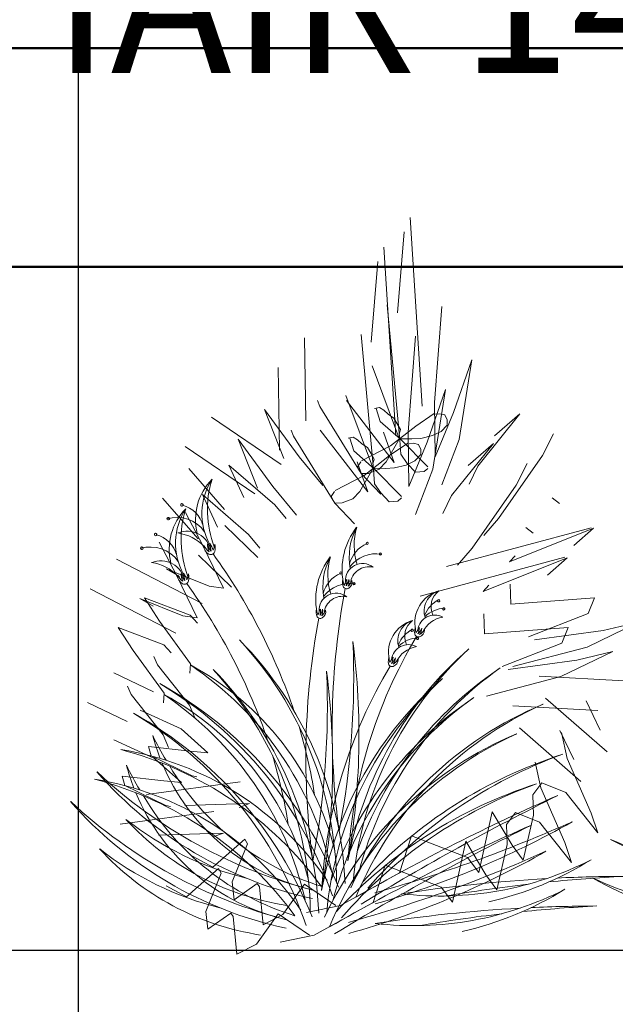
# Model space of a CAD drawing. Units: inches. Extents: x 89 to 490, y -59 to 378.
# Tile 3 of 20: x 275 to 300, y -26 to 15. Entities that reach past the tile are written whole.
import ezdxf

# ---------------------------------------------------------------- set-up
doc = ezdxf.new("R2010")
doc.units = ezdxf.units.IN
doc.header["$MEASUREMENT"] = 0
for name, color, linetype, lineweight in [('A-ANNO-DIMS', 2, 'Continuous', 18), ('L-PLNT', 94, 'Continuous', 18), ('L-PLNT-EDGE', 31, 'Continuous', 25), ('Outer Walls', 12, 'Continuous', 50)]:
    doc.layers.add(name, color=color, linetype=linetype, lineweight=lineweight)
doc.layers.add('fl', color=73, linetype='Continuous', lineweight=9, true_color=0xa3d166)
doc.styles.get("Standard").update_dxf_attribs({"font": 'arial.ttf'})
doc.dimstyles.get("Standard").update_dxf_attribs({"dimtxt": 6, "dimasz": 4, "dimexe": 3, "dimexo": 3, "dimgap": 0.09, "dimtad": 0, "dimtih": 1, "dimtoh": 1, "dimdec": 1, "dimzin": 0, "dimdsep": 46, "dimlunit": 3, "dimtxsty": 'Standard', "dimcen": 0.09, "dimadec": 0, "dimazin": 0, "dimtfac": 1, "dimtdec": 1, "dimtofl": 0, "dimtmove": 0, "dimatfit": 3, "dimfxl": 1, "dimtolj": 1, "dimtzin": 0, "dimarcsym": 0})

# ---------------------------------------------------------------- blocks, each defined once
blk = doc.blocks.new('Plantation')
at = {"layer": 'fl'}
for p, q in [((515.301, 41.637), (515.793, 33.876)), ((514.785, 37.717), (515.059, 41.049)), ((514.217, 40.419), (514.709, 32.658)), ((513.701, 36.499), (513.975, 39.831)), ((514.363, 38.042), (514.876, 32.478)), ((516.604, 37.97), (516.301, 34.022)), ((511.008, 33.275), (510.949, 36.687)), ((513.28, 36.824), (513.792, 31.26)), ((515.52, 36.752), (515.217, 32.804)), ((517.093, 33.612), (517.845, 35.777)), ((517.845, 35.777), (517.325, 32.502)), ((509.924, 32.057), (509.865, 35.469)), ((514.876, 32.478), (513.742, 35.536)), ((516.009, 32.394), (516.761, 34.559)), ((516.761, 34.559), (516.241, 31.284)), ((511.486, 34.101), (511.591, 33.862)), ((513.792, 31.26), (512.658, 34.318)), ((512.686, 34.103), (514.643, 31.559)), ((510.108, 31.721), (509.31, 33.735)), ((509.31, 33.735), (510.738, 31.791)), ((511.591, 33.862), (513.289, 31.1)), ((513.835, 33.771), (514.034, 33.811)), ((513.902, 33.777), (514.066, 33.248)), ((514.034, 33.811), (514.218, 33.705)), ((514.218, 33.705), (514.403, 33.544)), ((516.301, 34.022), (516.328, 31.787)), ((509.989, 31.478), (507.129, 33.424)), ((514.066, 33.248), (514.918, 32.499)), ((514.403, 33.544), (514.624, 33.384)), ((514.624, 33.384), (514.773, 33.15)), ((515.531, 33.055), (516.291, 33.567)), ((516.328, 31.787), (517.093, 33.612)), ((516.531, 33.563), (516.349, 33.541)), ((516.732, 33.512), (516.531, 33.563)), ((516.826, 33.313), (516.732, 33.512)), ((516.83, 33.095), (516.826, 33.313)), ((519.817, 33.559), (518.091, 31.41)), ((518.778, 32.649), (519.817, 33.559)), ((510.402, 32.883), (510.507, 32.644)), ((511.603, 32.885), (513.559, 30.341)), ((514.489, 32.241), (515.531, 33.055)), ((514.773, 33.15), (514.905, 32.915)), ((514.905, 32.915), (514.854, 32.714)), ((516.219, 32.665), (516.58, 32.835)), ((516.58, 32.835), (516.83, 33.095)), ((509.024, 30.503), (508.227, 32.517)), ((508.227, 32.517), (509.654, 30.573)), ((510.507, 32.644), (512.205, 29.882)), ((512.751, 32.553), (512.95, 32.593)), ((512.818, 32.559), (512.982, 32.03)), ((512.95, 32.593), (513.134, 32.487)), ((513.134, 32.487), (513.319, 32.326)), ((514.643, 31.559), (514.206, 32.799)), ((514.31, 31.576), (514.857, 32.514)), ((514.876, 32.478), (514.923, 31.896)), ((514.912, 32.533), (515.367, 32.523)), ((514.918, 32.499), (516.026, 31.37)), ((515.217, 32.804), (515.245, 30.569)), ((515.367, 32.523), (515.748, 32.548)), ((515.748, 32.548), (516.219, 32.665)), ((517.325, 32.502), (516.611, 30.63)), ((521.206, 32.731), (520.75, 31.841)), ((508.905, 30.26), (506.045, 32.206)), ((512.982, 32.03), (513.834, 31.281)), ((513.295, 31.617), (514.489, 32.241)), ((513.319, 32.326), (513.54, 32.166)), ((513.54, 32.166), (513.69, 31.932)), ((514.447, 31.837), (515.207, 32.349)), ((515.245, 30.569), (516.009, 32.394)), ((515.447, 32.345), (515.266, 32.323)), ((515.648, 32.294), (515.447, 32.345)), ((515.743, 32.095), (515.648, 32.294)), ((515.746, 31.877), (515.743, 32.095)), ((518.733, 32.341), (517.008, 30.192)), ((517.695, 31.431), (518.733, 32.341)), ((510.738, 31.791), (511.702, 30.609)), ((513.405, 31.023), (514.447, 31.837)), ((513.69, 31.932), (513.821, 31.697)), ((513.821, 31.697), (513.77, 31.496)), ((514.923, 31.896), (515.184, 31.518)), ((515.135, 31.447), (515.496, 31.617)), ((515.496, 31.617), (515.746, 31.877)), ((520.75, 31.841), (518.943, 29.251)), ((506.196, 31.305), (507.662, 29.625)), ((508.462, 30.109), (507.833, 31.449)), ((507.833, 31.449), (509.736, 29.812)), ((513.559, 30.341), (513.122, 31.581)), ((513.273, 31.576), (513.131, 31.373)), ((513.131, 31.373), (513.281, 31.103)), ((513.226, 30.358), (513.773, 31.296)), ((513.59, 31.108), (514.024, 31.279)), ((513.792, 31.26), (513.839, 30.678)), ((513.828, 31.315), (514.283, 31.305)), ((513.834, 31.281), (514.942, 30.152)), ((514.024, 31.279), (514.31, 31.576)), ((514.283, 31.305), (514.664, 31.33)), ((514.664, 31.33), (515.135, 31.447)), ((515.184, 31.518), (515.518, 31.16)), ((516.241, 31.284), (515.527, 29.412)), ((515.881, 31.184), (516.024, 31.314)), ((518.091, 31.41), (517.728, 30.668)), ((520.122, 31.513), (519.667, 30.623)), ((512.211, 30.399), (513.405, 31.023)), ((513.281, 31.103), (513.59, 31.108)), ((513.289, 31.1), (514.096, 30.253)), ((515.518, 31.16), (515.881, 31.184)), ((509.654, 30.573), (510.618, 29.391)), ((513.839, 30.678), (514.1, 30.3)), ((519.667, 30.623), (517.859, 28.033)), ((505.113, 30.087), (506.578, 28.407)), ((507.378, 28.891), (506.749, 30.231)), ((506.749, 30.231), (508.652, 28.594)), ((512.189, 30.358), (512.047, 30.155)), ((512.047, 30.155), (512.197, 29.885)), ((512.506, 29.89), (512.94, 30.061)), ((512.94, 30.061), (513.226, 30.358)), ((514.1, 30.3), (514.434, 29.942)), ((514.797, 29.966), (514.941, 30.096)), ((517.008, 30.192), (516.644, 29.45)), ((521.15, 30.104), (521.45, 29.871)), ((509.736, 29.812), (510.193, 29.245)), ((512.197, 29.885), (512.506, 29.89)), ((512.205, 29.882), (513.012, 29.035)), ((514.434, 29.942), (514.797, 29.966)), ((506.78, 28.107), (506.052, 29.492)), ((518.943, 29.251), (518.335, 28.55)), ((507.674, 28.964), (509.032, 27.649)), ((522.753, 28.872), (516.796, 27.271)), ((519.393, 27.468), (522.846, 28.85)), ((520.066, 28.886), (520.366, 28.653)), ((522.846, 28.85), (522.043, 28.142)), ((508.652, 28.594), (509.109, 28.027)), ((505.696, 26.889), (504.968, 28.274)), ((507.617, 26.386), (506.78, 28.107)), ((517.859, 28.033), (517.251, 27.332)), ((506.742, 25.747), (503.21, 27.571)), ((506.591, 27.746), (507.948, 26.431)), ((521.669, 27.654), (515.712, 26.053)), ((518.309, 26.25), (521.762, 27.632)), ((519.627, 27.719), (519.393, 27.468)), ((521.762, 27.632), (520.959, 26.924)), ((505.802, 26.859), (505.256, 27.18)), ((505.256, 27.18), (507.031, 26.463)), ((506.533, 25.168), (505.696, 26.889)), ((505.658, 24.529), (502.126, 26.353)), ((507.031, 26.463), (507.617, 26.386)), ((518.543, 26.501), (518.309, 26.25)), ((519.424, 26.545), (519.452, 25.72)), ((504.718, 25.641), (504.172, 25.962)), ((504.172, 25.962), (505.947, 25.245)), ((504.989, 25.032), (504.373, 25.984)), ((504.373, 25.984), (506.245, 25.27)), ((519.452, 25.72), (522.895, 25.983)), ((522.895, 25.983), (522.625, 25.342)), ((505.947, 25.245), (506.533, 25.168)), ((506.245, 25.27), (506.548, 24.94)), ((518.34, 25.327), (518.368, 24.502)), ((522.625, 25.342), (520.178, 24.384)), ((503.905, 23.814), (503.289, 24.766)), ((503.289, 24.766), (505.161, 24.052)), ((506.264, 23.277), (504.989, 25.032)), ((518.368, 24.502), (521.811, 24.765)), ((521.811, 24.765), (521.541, 24.124)), ((524.733, 24.997), (522.589, 23.962)), ((523.242, 24.639), (524.733, 24.997)), ((520.423, 24.257), (523.242, 24.639)), ((505.161, 24.052), (505.464, 23.722)), ((521.541, 24.124), (519.094, 23.166)), ((522.589, 23.962), (519.528, 23.16)), ((505.18, 22.059), (503.905, 23.814)), ((504.905, 23.231), (504.747, 23.566)), ((523.649, 23.779), (521.505, 22.744)), ((522.159, 23.421), (523.649, 23.779)), ((506.225, 21.574), (504.905, 23.231)), ((506.229, 22.887), (506.264, 23.277)), ((519.339, 23.039), (522.159, 23.421)), ((503.112, 22.9), (504.741, 22.12)), ((521.505, 22.744), (518.444, 21.942)), ((520.615, 22.763), (524.11, 22.574)), ((503.821, 22.013), (503.664, 22.348)), ((505.141, 20.356), (503.821, 22.013)), ((505.145, 21.669), (505.18, 22.059)), ((502.028, 21.682), (503.657, 20.902)), ((506.437, 21.047), (506.225, 21.574)), ((519.531, 21.545), (523.026, 21.356)), ((520.88, 21.852), (523.413, 19.651)), ((522.553, 21.742), (523.129, 20.547)), ((505.87, 20.59), (504.191, 21.359)), ((505.354, 19.829), (505.141, 20.356)), ((506.973, 19.607), (505.87, 20.59)), ((519.797, 20.634), (522.329, 18.433)), ((521.469, 20.524), (522.045, 19.329)), ((521.528, 20.443), (521.759, 19.382)), ((504.786, 19.372), (503.107, 20.141)), ((504.644, 19.479), (504.533, 19.864)), ((504.533, 19.864), (506.241, 19.679)), ((506.324, 18.661), (504.644, 19.479)), ((506.241, 19.679), (506.973, 19.607)), ((505.889, 18.389), (504.786, 19.372)), ((520.444, 19.225), (520.675, 18.164)), ((521.759, 19.382), (522.759, 17.131)), ((503.56, 18.261), (503.449, 18.646)), ((503.449, 18.646), (505.157, 18.461)), ((506.52, 18.619), (506.324, 18.661)), ((505.241, 17.443), (503.56, 18.261)), ((504.456, 17.894), (508.306, 18.41)), ((505.157, 18.461), (505.889, 18.389)), ((520.724, 18.374), (520.352, 17.875)), ((521.71, 17.97), (520.724, 18.374)), ((520.352, 17.875), (520.38, 17.05)), ((520.675, 18.164), (521.675, 15.913)), ((523.03, 16.314), (521.71, 17.97)), ((505.436, 17.401), (505.241, 17.443)), ((507.725, 17.493), (506.026, 17.435)), ((508.696, 17.527), (507.725, 17.493)), ((508.264, 17.366), (508.696, 17.527)), ((503.372, 16.676), (507.222, 17.192)), ((518.674, 17.186), (518.127, 14.688)), ((519.499, 15.805), (518.674, 17.186)), ((519.64, 17.156), (519.268, 16.657)), ((520.626, 16.752), (519.64, 17.156)), ((520.38, 17.05), (519.957, 15.188)), ((522.759, 17.131), (523.03, 16.314)), ((519.268, 16.657), (519.296, 15.832)), ((521.946, 15.096), (520.626, 16.752)), ((506.642, 16.275), (504.942, 16.217)), ((507.613, 16.309), (506.642, 16.275)), ((507.181, 16.148), (507.613, 16.309)), ((508.503, 16.062), (507.182, 14.898)), ((507.98, 14.294), (508.607, 15.871)), ((508.607, 15.871), (508.503, 16.062)), ((515.353, 16.198), (514.87, 14.674)), ((517.668, 15.305), (515.353, 16.198)), ((517.59, 15.968), (517.043, 13.47)), ((518.415, 14.587), (517.59, 15.968)), ((519.296, 15.832), (518.873, 13.97)), ((519.957, 15.188), (519.499, 15.805)), ((521.675, 15.913), (521.946, 15.096)), ((507.182, 14.898), (506.34, 15.356)), ((518.127, 14.688), (517.668, 15.305)), ((507.42, 14.844), (506.098, 13.68)), ((506.896, 13.076), (507.523, 14.653)), ((507.523, 14.653), (507.42, 14.844)), ((514.87, 14.674), (512.437, 13.328)), ((514.269, 14.98), (513.786, 13.456)), ((516.585, 14.087), (514.269, 14.98)), ((518.873, 13.97), (518.415, 14.587)), ((508.054, 13.567), (507.98, 14.294)), ((509.003, 14.231), (508.054, 13.567)), ((509.105, 14.089), (509.003, 14.231)), ((510.949, 14.2), (510.068, 12.955)), ((512.243, 13.321), (510.949, 14.2)), ((506.098, 13.68), (505.256, 14.138)), ((509.255, 12.538), (509.105, 14.089)), ((517.043, 13.47), (516.585, 14.087)), ((513.786, 13.456), (511.353, 12.11)), ((506.97, 12.349), (506.896, 13.076)), ((507.919, 13.013), (506.97, 12.349)), ((508.022, 12.871), (507.919, 13.013)), ((509.865, 12.982), (508.984, 11.737)), ((511.159, 12.103), (509.865, 12.982)), ((512.437, 13.328), (511.037, 13.037)), ((508.172, 11.32), (508.022, 12.871)), ((510.068, 12.955), (509.255, 12.538)), ((511.353, 12.11), (509.953, 11.819)), ((508.984, 11.737), (508.172, 11.32))]:
    blk.add_line(p, q, dxfattribs=at)
for centre, radius, start, end in [((508.843, 29.202), 2.375, 135.5632, 193.7293), ((509.331, 29.452), 2.601, 147.096, 209.2874), ((511.183, 29.607), 4.227, 162.6858, 201.1197), ((507.76, 27.984), 2.375, 135.5632, 193.7293), ((508.247, 28.234), 2.601, 147.096, 209.2874), ((505.909, 29.813), 0.053, 11.802, 191.802), ((505.909, 29.813), 0.053, 191.802, 11.802), ((510.099, 28.389), 4.227, 162.6858, 201.1197), ((505.648, 28.67), 1.163, 13.7128, 76.1437), ((505.341, 29.246), 0.053, 11.802, 191.802), ((505.688, 27.88), 1.416, 35.6636, 106.404), ((505.341, 29.246), 0.053, 191.802, 11.802), ((515.355, 27.138), 2.854, 142.1725, 190.5866), ((515.393, 27.66), 2.6, 151.8051, 190.4904), ((515.605, 28.157), 2.608, 163.721, 197.6936), ((504.825, 28.595), 0.053, 11.802, 191.802), ((504.825, 28.595), 0.053, 191.802, 11.802), ((504.564, 27.452), 1.163, 13.7128, 76.1437), ((506.121, 27.716), 1.01, 11.1862, 111.7493), ((505.463, 26.791), 1.886, 44.0209, 81.3627), ((504.257, 28.028), 0.053, 11.802, 191.802), ((504.605, 26.662), 1.416, 35.6636, 106.404), ((504.257, 28.028), 0.053, 191.802, 11.802), ((507.154, 28.091), 0.334, 172.3781, 246.6066), ((507.443, 28.435), 0.689, 205.7422, 233.1344), ((507.608, 28.188), 0.654, 178.723, 207.7572), ((507.764, 28.455), 0.848, 197.3111, 219.7508), ((506.427, 27.721), 0.803, 16.3461, 37.9549), ((508.569, 28.321), 1.513, 184.0141, 195.6693), ((506.064, 28.381), 1.213, 339.0728, 350.8866), ((506.59, 28.04), 0.688, 348.1534, 12.4334), ((514.008, 27.069), 1.243, 113.1986, 165.1488), ((513.532, 28.225), 0.0459, 354.4108, 174.4108), ((513.532, 28.225), 0.0459, 174.4108, 354.4108), ((507.094, 27.943), 0.175, 245.3588, 345.3239), ((487.153, 13.359), 24.696, 18.7875, 35.7756), ((514.271, 25.92), 2.854, 142.1725, 190.5866), ((514.309, 26.442), 2.6, 151.8051, 190.4904), ((514.521, 26.939), 2.608, 163.721, 197.6936), ((513.923, 26.417), 1.386, 81.8677, 142.4931), ((514.073, 27.791), 0.0459, 174.4108, 354.4108), ((514.073, 27.791), 0.0459, 354.4108, 174.4108), ((505.037, 26.498), 1.01, 11.1862, 111.7493), ((504.379, 25.573), 1.886, 44.0209, 81.3627), ((513.34, 26.698), 0.701, 51.1297, 184.5825), ((513.596, 26.513), 0.754, 75.8945, 175.0168), ((506.07, 26.873), 0.334, 172.3781, 246.6066), ((506.359, 27.217), 0.689, 205.7422, 233.1344), ((506.524, 26.97), 0.654, 178.723, 207.7572), ((506.68, 27.237), 0.848, 197.3111, 219.7508), ((505.343, 26.503), 0.803, 16.3461, 37.9549), ((507.485, 27.103), 1.513, 184.0141, 195.6693), ((504.98, 27.163), 1.213, 339.0728, 350.8866), ((505.506, 26.822), 0.688, 348.1534, 12.4334), ((512.924, 25.851), 1.243, 113.1986, 165.1488), ((512.448, 27.007), 0.0459, 354.4108, 174.4108), ((512.448, 27.007), 0.0459, 174.4108, 354.4108), ((513.283, 26.378), 0.694, 148.2579, 169.8667), ((511.385, 26.693), 1.308, 350.5435, 2.1987), ((512.065, 26.883), 0.733, 326.462, 348.9017), ((512.224, 26.669), 0.565, 338.4556, 7.4897), ((506.01, 26.725), 0.175, 245.3588, 345.3239), ((486.07, 12.141), 24.696, 18.7875, 35.7756), ((512.839, 25.199), 1.386, 81.8677, 142.4931), ((543.585, 20.607), 31.492, 169.4573, 187.7209), ((513.113, 26.637), 0.595, 173.7794, 198.0594), ((513.533, 26.979), 1.049, 195.3262, 207.14), ((512.688, 26.507), 0.151, 200.8889, 300.854), ((512.342, 26.897), 0.596, 313.0784, 340.4706), ((512.623, 26.628), 0.289, 299.6062, 13.8346), ((512.989, 26.573), 0.0459, 174.4108, 354.4108), ((512.989, 26.573), 0.0459, 354.4108, 174.4108), ((512.256, 25.48), 0.701, 51.1297, 184.5825), ((512.512, 25.295), 0.754, 75.8945, 175.0168), ((516.862, 24.955), 1.368, 105.8634, 192.367), ((516.74, 25.445), 0.863, 106.9799, 199.184), ((516.952, 25.627), 0.793, 125.7722, 206.2024), ((512.199, 25.16), 0.694, 148.2579, 169.8667), ((510.302, 25.475), 1.308, 350.5435, 2.1987), ((510.981, 25.665), 0.733, 326.462, 348.9017), ((511.14, 25.451), 0.565, 338.4556, 7.4897), ((517.047, 24.803), 1.243, 116.6992, 157.9158), ((516.828, 24.183), 1.386, 94.6451, 131.584), ((516.475, 25.869), 0.0459, 162.351, 342.351), ((516.475, 25.869), 0.0459, 342.351, 162.351), ((516.686, 25.529), 0.0459, 162.351, 342.351), ((516.686, 25.529), 0.0459, 342.351, 162.351), ((542.502, 19.389), 31.492, 169.4573, 187.7209), ((512.029, 25.419), 0.595, 173.7794, 198.0594), ((512.449, 25.761), 1.049, 195.3262, 207.14), ((511.605, 25.289), 0.151, 200.8889, 300.854), ((511.258, 25.679), 0.596, 313.0784, 340.4706), ((511.539, 25.41), 0.289, 299.6062, 13.8346), ((516.312, 24.583), 0.696, 61.775, 172.7958), ((516.846, 24.061), 1.154, 100.1929, 154.0707), ((515.779, 23.737), 1.368, 105.8634, 192.367), ((515.657, 24.227), 0.863, 106.9799, 199.184), ((515.868, 24.409), 0.793, 125.7722, 206.2024), ((516.082, 24.567), 0.595, 161.7196, 185.9995), ((516.564, 24.814), 1.049, 183.2663, 195.0802), ((516.194, 24.278), 0.694, 136.198, 157.8068), ((514.404, 24.983), 1.308, 338.4836, 350.1389), ((515.108, 25.027), 0.733, 314.4022, 336.8418), ((515.219, 24.784), 0.565, 326.3958, 355.4299), ((532.929, 14.051), 20.216, 149.2128, 176.849), ((515.963, 23.585), 1.243, 116.6992, 157.9158), ((515.744, 22.965), 1.386, 94.6451, 131.584), ((515.391, 24.651), 0.0459, 162.351, 342.351), ((515.391, 24.651), 0.0459, 342.351, 162.351), ((515.64, 24.528), 0.151, 188.8291, 288.7942), ((515.602, 24.311), 0.0459, 162.351, 342.351), ((515.602, 24.311), 0.0459, 342.351, 162.351), ((515.601, 24.661), 0.289, 287.5463, 1.7748), ((515.382, 24.982), 0.596, 301.0185, 328.4108), ((497.355, 14.09), 14.921, 0.703, 42.9608), ((497.433, 13.602), 15.201, 2.3901, 44.5084), ((478.991, 22.735), 33.989, 349.2183, 2.4529), ((483.302, 20.348), 29.894, 350.0105, 7.3826), ((515.228, 23.365), 0.696, 61.775, 172.7958), ((515.762, 22.843), 1.154, 100.1929, 154.0707), ((527.693, 12.415), 15.201, 130.9977, 169.5878), ((527.81, 12.895), 14.921, 132.5453, 174.8032), ((514.998, 23.349), 0.595, 161.7196, 185.9995), ((515.48, 23.596), 1.049, 183.2663, 195.0802), ((515.11, 23.06), 0.694, 136.198, 157.8068), ((513.32, 23.765), 1.308, 338.4836, 350.1389), ((514.024, 23.809), 0.733, 314.4022, 336.8418), ((514.135, 23.566), 0.565, 326.3958, 355.4299), ((498.551, 11.706), 13.856, 12.8419, 56.2195), ((500.549, 12.648), 12.017, 14.1577, 61.6464), ((531.845, 12.833), 20.216, 149.2128, 176.849), ((527.451, 10.46), 15.201, 123.7186, 160.4349), ((527.628, 10.922), 14.921, 125.2661, 165.1679), ((514.556, 23.31), 0.151, 188.8291, 288.7942), ((514.517, 23.443), 0.289, 287.5463, 1.7748), ((514.298, 23.764), 0.596, 301.0185, 328.4108), ((496.271, 12.872), 14.921, 0.703, 42.9608), ((496.35, 12.384), 15.201, 2.3901, 44.5084), ((477.907, 21.516), 33.989, 349.2183, 2.4529), ((482.218, 19.13), 29.894, 350.0105, 7.3826), ((496.888, 7.925), 16.642, 21.708, 60.8529), ((496.735, 8.477), 16.239, 18.8656, 59.433), ((526.61, 11.197), 15.201, 130.9977, 169.5878), ((526.726, 11.677), 14.921, 132.5453, 174.8032), ((497.468, 10.488), 13.856, 12.8419, 56.2195), ((499.465, 11.43), 12.017, 14.1577, 61.6464), ((526.367, 9.242), 15.201, 123.7186, 160.4349), ((526.544, 9.704), 14.921, 125.2661, 165.1679), ((526.606, 7.568), 15.201, 112.5744, 154.7193), ((526.869, 7.987), 14.921, 114.122, 157.6363), ((495.804, 6.707), 16.642, 21.708, 60.8529), ((495.651, 7.259), 16.239, 18.8656, 59.433), ((489.58, 14.392), 22.067, 9.068, 16.6817), ((513.284, 22.613), 8.88, 194.9574, 201.3849), ((516.385, 25.976), 12.977, 205.8333, 210.9541), ((525.522, 6.35), 15.201, 112.5744, 154.7193), ((525.785, 6.769), 14.921, 114.122, 157.6363), ((501.425, 7.255), 12.64, 34.1912, 81.04), ((499.608, 5.319), 14.911, 36.1662, 75.2917), ((488.496, 13.174), 22.067, 9.068, 16.6817), ((527.445, 1.272), 19.194, 107.7857, 137.2506), ((528.058, 1.531), 19.147, 109.7712, 139.1936), ((512.201, 21.395), 8.88, 194.9574, 201.3849), ((515.302, 24.758), 12.977, 205.8333, 210.9541), ((513.284, 22.613), 8.88, 202.7107, 257.3947), ((514.919, 24.664), 11.042, 210.5234, 252.7528), ((516.372, 33.787), 20.466, 226.9943, 255.7863), ((514.692, 29.576), 16.324, 221.2139, 257.9277), ((500.341, 6.037), 12.64, 34.1912, 81.04), ((498.524, 4.101), 14.911, 36.1662, 75.2917), ((526.361, 0.054), 19.194, 107.7857, 137.2506), ((526.975, 0.313), 19.147, 109.7712, 139.1936), ((512.201, 21.395), 8.88, 202.7107, 257.3947), ((513.836, 23.446), 11.042, 210.5234, 252.7528), ((554.444, -58.066), 82.807, 113.53444, 119.97645), ((569.304, -78.592), 107.696, 116.42332, 121.34648), ((515.288, 32.569), 20.466, 226.9943, 255.7863), ((513.608, 28.358), 16.324, 221.2139, 257.9277), ((511.723, 27.2), 13.137, 231.8384, 256.0141), ((511.953, 24.524), 11.325, 222.5197, 261.2503), ((553.36, -59.284), 82.807, 113.53444, 119.97645), ((568.22, -79.81), 107.696, 116.42332, 121.34648), ((498.147, 70.245), 58.541, 285.56, 294.0219), ((503.886, 48.785), 36.77, 285.7446, 299.4741), ((540.511, 48.666), 36.77, 242.5259, 256.2554), ((545.497, 70.313), 58.541, 247.9781, 256.44), ((510.64, 25.982), 13.137, 231.8384, 256.0141), ((510.869, 23.306), 11.325, 222.5197, 261.2503), ((497.063, 69.027), 58.541, 285.56, 294.0219), ((502.802, 47.567), 36.77, 285.7446, 299.4741), ((516.534, 27.42), 13.704, 263.3334, 297.0085), ((515.381, 27.161), 14.044, 282.9751, 301.6856), ((524.217, -45.831), 60.356, 93.13909, 98.84209), ((527.051, -45.8), 60.398, 96.55624, 99.79042), ((527.051, -45.8), 60.398, 92.82762, 95.73925), ((524.217, -45.831), 60.356, 90.13814, 92.7056), ((529.777, 26.654), 14.044, 240.3144, 259.0249), ((528.616, 26.873), 13.704, 244.9915, 278.6666), ((515.45, 26.202), 13.704, 263.3334, 297.0085), ((514.297, 25.943), 14.044, 282.9751, 301.6856), ((523.133, -47.049), 60.356, 93.13909, 98.84209), ((525.967, -47.018), 60.398, 96.55624, 99.79042), ((525.967, -47.018), 60.398, 92.82762, 95.73925), ((523.133, -47.049), 60.356, 90.13814, 92.7056)]:
    blk.add_arc(centre, radius, start, end, dxfattribs=at)
blk = doc.blocks.new('*D28')
at = {"layer": 'A-ANNO-DIMS', "color": 0, "lineweight": -2, "transparency": 16777216}
for p, q in [((326.431, 33.398), (324.379, 33.398)), ((327.379, 29.398), (327.379, 23.72)), ((326.431, 19.72), (324.379, 19.72)), ((327.379, 19.72), (327.379, 15.72)), ((327.379, 15.72), (323.379, 15.72))]:
    blk.add_line(p, q, dxfattribs=at)
at = {"layer": 'A-ANNO-DIMS', "color": 0, "transparency": 16777216}
for points in [[(326.712, 29.398), (328.046, 29.398), (327.379, 33.398)], [(326.712, 23.72), (328.046, 23.72), (327.379, 19.72)]]:
    blk.add_solid(points, dxfattribs=at)
at = {"layer": 'Defpoints', "color": 0, "transparency": 16777216}
for p in [(329.431, 33.398), (327.379, 19.72), (329.431, 19.72)]:
    blk.add_point(p, dxfattribs=at)
at = {"layer": 'A-ANNO-DIMS', "color": 0, "transparency": 16777216, "insert": (294.517, 15.72), "char_height": 6, "attachment_point": 5}
blk.add_mtext('\\A1;CHAIR 14 TYP.', dxfattribs=at)
blk = doc.blocks.new('*D46')
at = {"layer": 'A-ANNO-DIMS', "color": 0, "lineweight": -2, "transparency": 16777216}
for p, q in [((277.443, -27.866), (277.443, -53.11)), ((445.739, -27.866), (445.739, -53.11)), ((281.443, -50.11), (332.892, -50.11)), ((441.739, -50.11), (390.289, -50.11))]:
    blk.add_line(p, q, dxfattribs=at)
at = {"layer": 'A-ANNO-DIMS', "color": 0, "transparency": 16777216}
for points in [[(281.443, -49.443), (281.443, -50.777), (277.443, -50.11)], [(441.739, -49.443), (441.739, -50.777), (445.739, -50.11)]]:
    blk.add_solid(points, dxfattribs=at)
at = {"layer": 'Defpoints', "color": 0, "transparency": 16777216}
for p in [(277.443, -24.866), (445.739, -24.866), (445.739, -50.11)]:
    blk.add_point(p, dxfattribs=at)
at = {"layer": 'A-ANNO-DIMS', "color": 0, "transparency": 16777216, "insert": (361.591, -50.11), "char_height": 6, "attachment_point": 5}
blk.add_mtext('\\A1;PLANTING 168', dxfattribs=at)
blk = doc.blocks.new('*D48')
at = {"layer": 'A-ANNO-DIMS', "color": 0, "lineweight": -2, "transparency": 16777216}
for p, q in [((127.441, 10.741), (127.441, -49.809)), ((459.441, -29.659), (459.441, -49.809)), ((131.441, -46.809), (286.756, -46.809)), ((455.441, -46.809), (300.127, -46.809))]:
    blk.add_line(p, q, dxfattribs=at)
at = {"layer": 'A-ANNO-DIMS', "color": 0, "transparency": 16777216}
for points in [[(131.441, -46.143), (131.441, -47.476), (127.441, -46.809)], [(455.441, -46.143), (455.441, -47.476), (459.441, -46.809)]]:
    blk.add_solid(points, dxfattribs=at)
at = {"layer": 'Defpoints', "color": 0, "transparency": 16777216}
for p in [(127.441, 13.741), (459.441, -26.659), (459.441, -46.809)]:
    blk.add_point(p, dxfattribs=at)
at = {"layer": 'A-ANNO-DIMS', "color": 0, "transparency": 16777216, "insert": (293.441, -46.809), "char_height": 6, "attachment_point": 5}
blk.add_mtext('\\A1;332', dxfattribs=at)
blk = doc.blocks.new('*D74')
at = {"layer": 'A-ANNO-DIMS', "color": 0, "lineweight": -2, "transparency": 16777216}
for p, q in [((249.441, 341.741), (249.441, -49.809)), ((277.753, 341.347), (277.753, -49.809)), ((253.441, -46.809), (253.912, -46.809)), ((273.753, -46.809), (273.283, -46.809))]:
    blk.add_line(p, q, dxfattribs=at)
at = {"layer": 'A-ANNO-DIMS', "color": 0, "transparency": 16777216}
for points in [[(253.441, -46.143), (253.441, -47.476), (249.441, -46.809)], [(273.753, -46.143), (273.753, -47.476), (277.753, -46.809)]]:
    blk.add_solid(points, dxfattribs=at)
at = {"layer": 'Defpoints', "color": 0, "transparency": 16777216}
for p in [(249.441, 344.741), (277.753, 344.347), (277.753, -46.809)]:
    blk.add_point(p, dxfattribs=at)
at = {"layer": 'A-ANNO-DIMS', "color": 0, "transparency": 16777216, "insert": (263.597, -46.809), "char_height": 6, "attachment_point": 5}
blk.add_mtext('\\A1;28.31', dxfattribs=at)

msp = doc.modelspace()

# ---------------------------------------------------------------- linework, layer by layer
at = {"layer": 'L-PLNT-EDGE'}
msp.add_line((459.4414, -23.3886), (265.4414, -23.3886), dxfattribs=at)
at = {"layer": 'Outer Walls'}
msp.add_line((270.4414, 13.7413), (450.4414, 13.7413), dxfattribs=at)
msp.add_lwpolyline([(214.6478, 67.7413), (265.4414, 67.7413), (265.4414, 4.7413), (459.4414, 4.7413), (459.4414, 353.7413), (127.4414, 353.7413), (127.4414, 13.7413)], dxfattribs=at)

# ---------------------------------------------------------------- block references
at = {"layer": 'L-PLNT'}
msp.add_blockref('Plantation', (-223.8856, -34.8668), dxfattribs=at)

# ---------------------------------------------------------------- dimensions: what is measured, and where the dimension line sits
at = {"layer": 'A-ANNO-DIMS'}
for base, p1, p2, override, picture, middle in [((277.7535, -46.8094), (249.4414, 344.7413), (277.7535, 344.3468), {"dimdec": 2, "dimlfac": 1, "dimrnd": 0, "dimzin": 0, "dimdsep": 46, "dimlunit": 2}, '*D74', (263.5974, -46.8094)), ((459.4414, -46.8094), (127.4414, 13.7413), (459.4414, -26.6594), {"dimdec": 0, "dimlfac": 1, "dimrnd": 0, "dimzin": 0, "dimdsep": 46, "dimlunit": 2}, '*D48', (293.4414, -46.8094))]:
    dim = msp.add_linear_dim(base=base, p1=p1, p2=p2, dimstyle='Standard', override=override, dxfattribs=at)
    dim.commit()
    dim.dimension.update_dxf_attribs({"geometry": picture, "text_midpoint": middle})
dim = msp.add_linear_dim(base=(327.3791, 19.7198), p1=(329.4308, 33.3978), p2=(329.4308, 19.7198), angle=270, text='CHAIR <> TYP.', dimstyle='Standard', override={"dimdec": 0, "dimlfac": 1, "dimrnd": 0, "dimzin": 0, "dimdsep": 46, "dimlunit": 2}, dxfattribs=at)
dim.commit()
dim.dimension.update_dxf_attribs({"geometry": '*D28', "text_midpoint": (294.517, 15.7198)})
dim = msp.add_linear_dim(base=(445.7386, -50.11), p1=(277.443, -24.8656), p2=(445.7386, -24.8656), text='PLANTING <>', dimstyle='Standard', override={"dimdec": 0, "dimlfac": 1, "dimrnd": 0, "dimzin": 0, "dimdsep": 46, "dimlunit": 2}, dxfattribs=at)
dim.commit()
dim.dimension.update_dxf_attribs({"geometry": '*D46', "text_midpoint": (361.5908, -50.11)})

doc.saveas('drawing.dxf')
